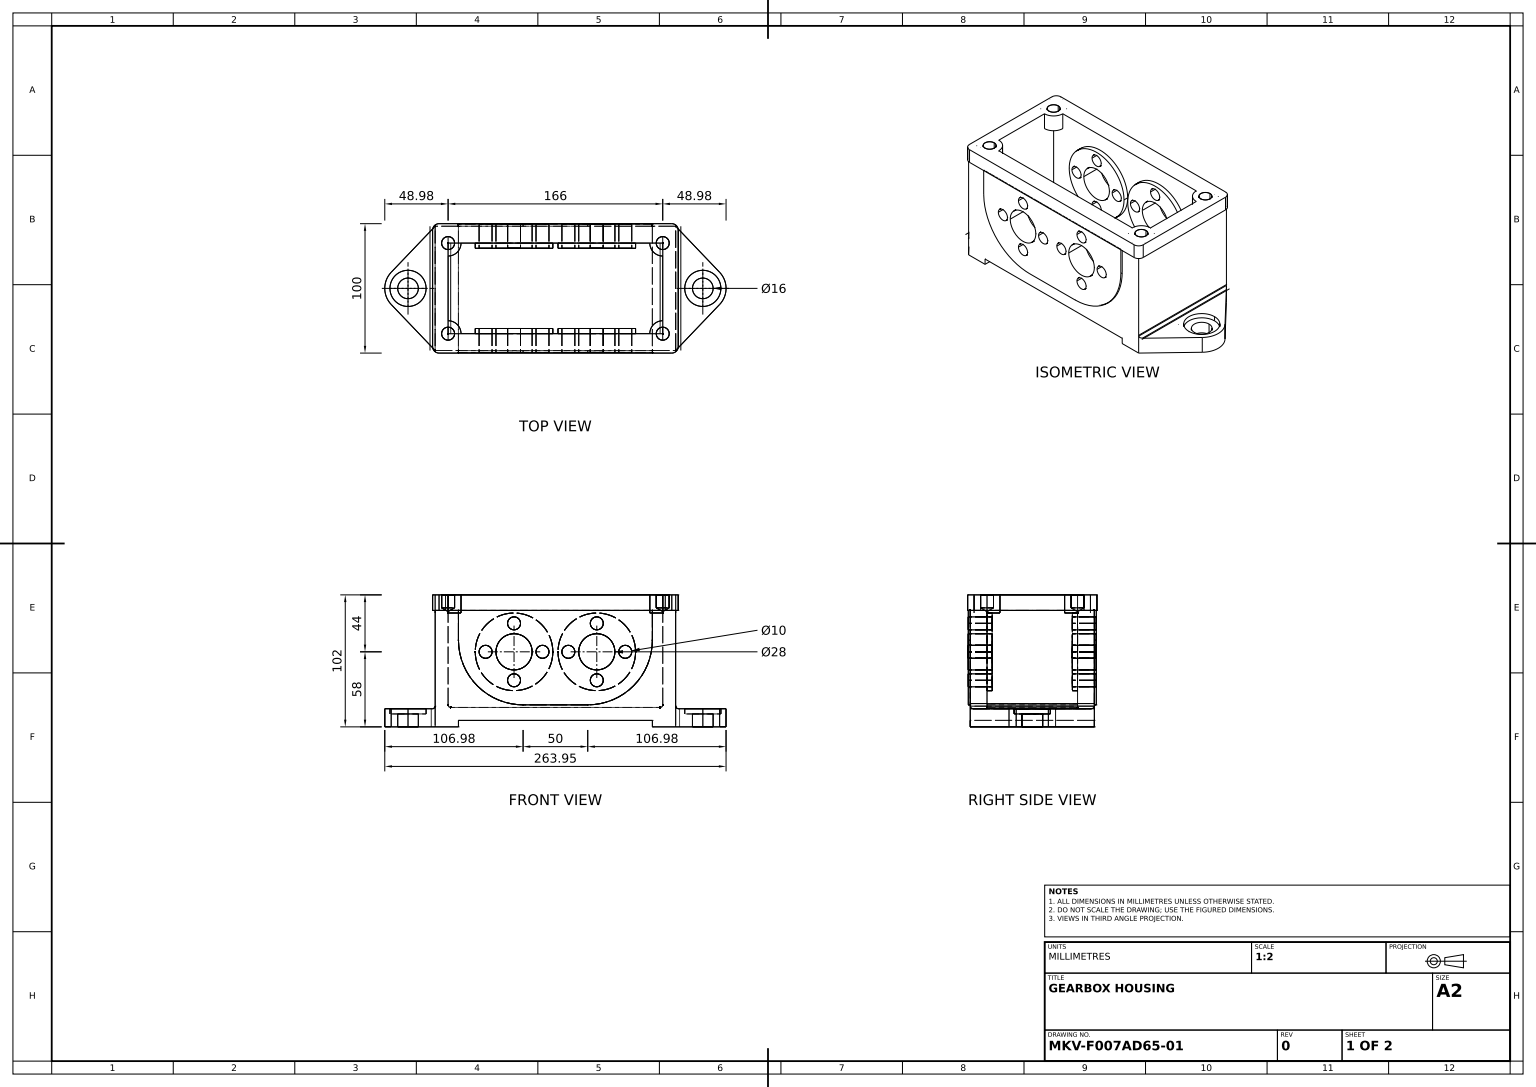
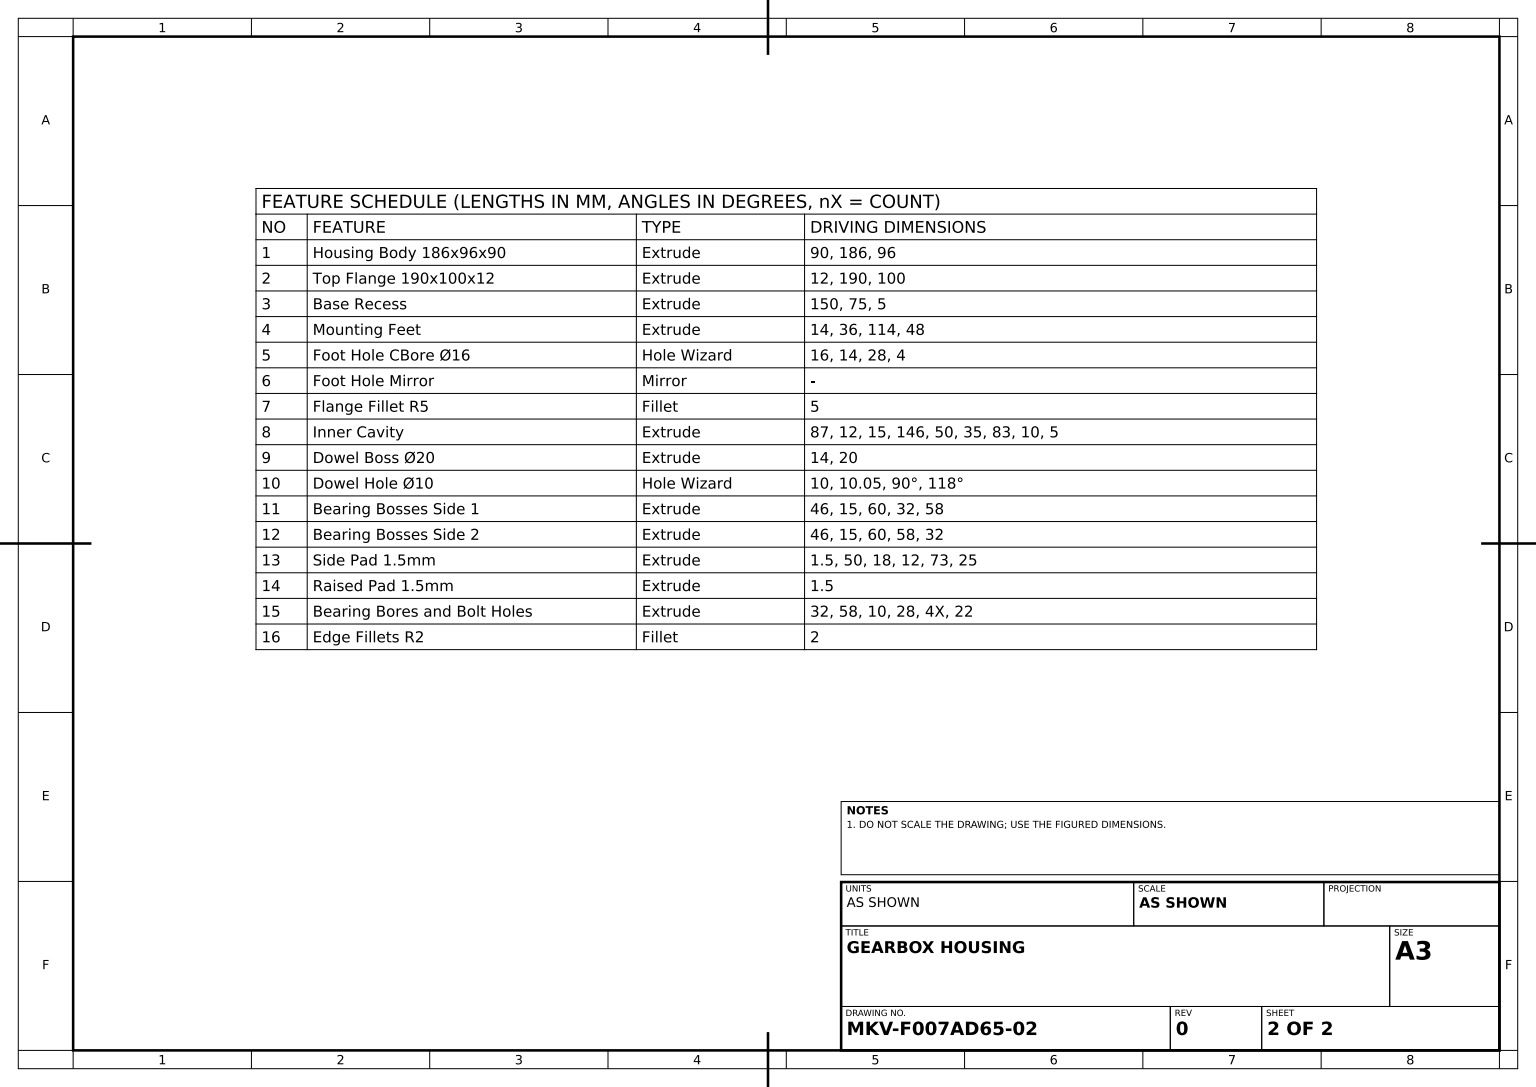
from build123d import *

# Parameters (mm, degrees)
HOUSING_BODY_SKETCH_W                   = 186
HOUSING_BODY_SKETCH_H                   = 96
HOUSING_BODY_186X96X90_DEPTH            = 90
TOP_FLANGE_SKETCH_W                     = 190
TOP_FLANGE_SKETCH_H                     = 100
TOP_FLANGE_190X100X12_DEPTH             = 12
BASE_RECESS_SKETCH_W                    = 150
BASE_RECESS_SKETCH_H                    = 5
BASE_RECESS_DEPTH                       = 171.390727447
MOUNTING_FEET_DEPTH                     = 14
FOOT_HOLE_CBORE_16_D                    = 16
FOOT_HOLE_CBORE_16_CBORE_D              = 28
FOOT_HOLE_CBORE_16_CBORE_DEPTH          = 4
FLANGE_FILLET_R5_R                      = 5
INNER_CAVITY_DEPTH                      = 87
DOWEL_BOSS_SKETCH_R                     = 10
DOWEL_BOSS_20_DEPTH                     = 14
DOWEL_HOLE_10_D                         = 10
DOWEL_HOLE_10_DEPTH                     = 10
DOWEL_HOLE_10_CSINK_D                   = 10.05
DOWEL_HOLE_10_CSINK_ANGLE               = 90
DOWEL_HOLE_10_TIP                       = 3.004303095
BEARING_BOSSES_SIDE_1_SKETCH_R          = 30
BEARING_BOSSES_SIDE_1_DEPTH             = 15
BEARING_START                           = -15
BEARING_BOSSES_SIDE_2_SKETCH_R          = 30
BEARING_BOSSES_SIDE_2_DEPTH             = 15
SIDE_PAD_1_5MM_DEPTH                    = 1.5
RAISED_START                            = 1.5
RAISED_PAD_1_5MM_DEPTH                  = 1.5
BEARING_BORES_AND_BOLT_HOLES_SKETCH_R   = 5
BEARING_BORES_AND_BOLT_HOLES_SKETCH_R_2 = 14
BEARING_BORES_AND_BOLT_HOLES_DEPTH      = 195.237612218
EDGE_FILLETS_R2_R                       = 2


with BuildPart() as part:
    # Housing Body Sketch → Housing Body 186x96x90 (new body)
    with BuildSketch(Plane(origin=(0, 0, 0), x_dir=(1, 0, 0), z_dir=(0, 1, 0))):
        Rectangle(HOUSING_BODY_SKETCH_W, HOUSING_BODY_SKETCH_H)
    extrude(amount=HOUSING_BODY_186X96X90_DEPTH)

    # Top Flange Sketch → Top Flange 190x100x12 (add)
    with BuildSketch(Plane(origin=(0, 90, 0), x_dir=(1, 0, 0), z_dir=(0, 1, 0))):
        Rectangle(TOP_FLANGE_SKETCH_W, TOP_FLANGE_SKETCH_H)
    extrude(amount=TOP_FLANGE_190X100X12_DEPTH)

    # Base Recess Sketch → Base Recess (cut, through all)
    with BuildSketch(Plane.XY.offset(48)):
        with Locations((0, 2.5)):
            Rectangle(BASE_RECESS_SKETCH_W, BASE_RECESS_SKETCH_H)
    extrude(amount=-BASE_RECESS_DEPTH, mode=Mode.SUBTRACT)

    # Mounting Feet Sketch → Mounting Feet (add)
    with BuildSketch(Plane.XZ):
        with BuildLine():
            Line((-127.008364611, 12.441159517), (-93, 48))
            Line((-93, 48), (-93, -48))
            Line((-93, -48), (-127.008364611, -12.441159517))
            ThreePointArc((-127.008364611, -12.441159517), (-132, 0), (-127.008364611, 12.441159517))
        make_face()
    mounting_feet = extrude(amount=-MOUNTING_FEET_DEPTH)

    # Foot Hole CBore Ø16 (through all)
    with Locations(Plane(origin=(0, 14, 0), x_dir=(1, 0, 0), z_dir=(0, 1, 0))):
        with Locations((-114, 0)):
            foot_hole_cbore_16 = CounterBoreHole(FOOT_HOLE_CBORE_16_D / 2, FOOT_HOLE_CBORE_16_CBORE_D / 2, FOOT_HOLE_CBORE_16_CBORE_DEPTH)

    # Foot Hole Mirror: Mounting Feet, Foot Hole CBore Ø16 across plane
    add(mounting_feet.mirror(Plane(origin=(0, 0, 0), x_dir=(0, 0, 1), z_dir=(1, 0, 0))))
    add(foot_hole_cbore_16.mirror(Plane(origin=(0, 0, 0), x_dir=(0, 0, 1), z_dir=(1, 0, 0))), mode=Mode.SUBTRACT)

    # Flange Fillet R5
    flange_fillet_r5_edges = [part.edges().sort_by_distance(p)[0] for p in [
        (95, 96, 50),
        (95, 96, -50),
        (-95, 96, -50),
        (-95, 96, 50),
    ]]
    fillet(flange_fillet_r5_edges, radius=FLANGE_FILLET_R5_R)

    # Inner Cavity Sketch → Inner Cavity (cut)
    with BuildSketch(Plane(origin=(0, 102, 0), x_dir=(1, 0, 0), z_dir=(0, 1, 0))):
        Polygon((-73, 35), (73, 35), (83, 35), (83, 25), (83, -25), (83, -35), (73, -35), (-73, -35), (-83, -35), (-83, -25), (-83, 25), (-83, 35), align=None)
    extrude(amount=-INNER_CAVITY_DEPTH, mode=Mode.SUBTRACT)

    # Dowel Boss Sketch → Dowel Boss Ø20 (add)
    with BuildSketch(Plane(origin=(0, 102, 0), x_dir=(1, 0, 0), z_dir=(0, 1, 0))):
        with Locations((-83, 35)):
            Circle(DOWEL_BOSS_SKETCH_R)
        with Locations((83, 35)):
            Circle(DOWEL_BOSS_SKETCH_R)
        with Locations((83, -35)):
            Circle(DOWEL_BOSS_SKETCH_R)
        with Locations((-83, -35)):
            Circle(DOWEL_BOSS_SKETCH_R)
    extrude(amount=-DOWEL_BOSS_20_DEPTH)

    # Dowel Hole Ø10
    with Locations(Plane(origin=(0, 102, 0), x_dir=(1, 0, 0), z_dir=(0, 1, 0))):
        with Locations((-83, -35), (-83, 35), (83, 35), (83, -35)):
            CounterSinkHole(DOWEL_HOLE_10_D / 2, DOWEL_HOLE_10_CSINK_D / 2, depth=DOWEL_HOLE_10_DEPTH, counter_sink_angle=DOWEL_HOLE_10_CSINK_ANGLE)
            with Locations((0, 0, -(DOWEL_HOLE_10_DEPTH + DOWEL_HOLE_10_TIP / 2))):  # 118° drill point
                Cone(0, DOWEL_HOLE_10_D / 2, DOWEL_HOLE_10_TIP, mode=Mode.SUBTRACT)

    # Bearing Bosses Side 1 Sketch → Bearing Bosses Side 1 (add)
    with BuildSketch(Plane.XY.offset(-46)):
        with Locations(Location((-32, 58, 0), (0, 0, 180))):
            Circle(BEARING_BOSSES_SIDE_1_SKETCH_R)
        with Locations(Location((32, 58, 0), (0, 0, 180))):
            Circle(BEARING_BOSSES_SIDE_1_SKETCH_R)
    extrude(amount=BEARING_BOSSES_SIDE_1_DEPTH)

    # Bearing Bosses Side 2 Sketch → Bearing Bosses Side 2 (add)
    with BuildSketch(Plane.XY.offset(46).offset(BEARING_START)):
        with Locations(Location((32, 58, 0), (0, 0, 180))):
            Circle(BEARING_BOSSES_SIDE_2_SKETCH_R)
        with Locations(Location((-32, 58, 0), (0, 0, 180))):
            Circle(BEARING_BOSSES_SIDE_2_SKETCH_R)
    extrude(amount=BEARING_BOSSES_SIDE_2_DEPTH)

    # Side Pad Sketch → Side Pad 1.5mm (add)
    with BuildSketch(Plane(origin=(0, 0, -48), x_dir=(-1, 0, 0), z_dir=(0, 0, -1))):
        with BuildLine():
            Line((-25, 17), (0, 17))
            Line((0, 17), (25, 17))
            ThreePointArc((25, 17), (60.355339059, 31.644660941), (75, 67))
            Line((75, 67), (75, 90))
            Line((75, 90), (-75, 90))
            Line((-75, 90), (-75, 67))
            ThreePointArc((-75, 67), (-60.355339059, 31.644660941), (-25, 17))
        make_face()
    extrude(amount=SIDE_PAD_1_5MM_DEPTH)

    # Raised Pad Sketch → Raised Pad 1.5mm (add)
    with BuildSketch(Plane.XY.offset(48).offset(RAISED_START)):
        with BuildLine():
            Line((75, 90), (75, 67))
            ThreePointArc((75, 67), (60.355339059, 31.644660941), (25, 17))
            Line((25, 17), (-25, 17))
            ThreePointArc((-25, 17), (-60.355339059, 31.644660941), (-75, 67))
            Line((-75, 67), (-75, 90))
            Line((-75, 90), (75, 90))
        make_face()
    extrude(amount=-RAISED_PAD_1_5MM_DEPTH)

    # Bearing Bores and Bolt Holes Sketch → Bearing Bores and Bolt Holes (cut, through all)
    with BuildSketch(Plane.XY.offset(49.5)):
        with Locations((-32, 80)):
            Circle(BEARING_BORES_AND_BOLT_HOLES_SKETCH_R)
        with Locations((32, 80)):
            Circle(BEARING_BORES_AND_BOLT_HOLES_SKETCH_R)
        with Locations((-32, 58)):
            Circle(BEARING_BORES_AND_BOLT_HOLES_SKETCH_R_2)
        with Locations((32, 58)):
            Circle(BEARING_BORES_AND_BOLT_HOLES_SKETCH_R_2)
        with Locations((-10, 58)):
            Circle(BEARING_BORES_AND_BOLT_HOLES_SKETCH_R)
        with Locations((-32, 36)):
            Circle(BEARING_BORES_AND_BOLT_HOLES_SKETCH_R)
        with Locations((-54, 58)):
            Circle(BEARING_BORES_AND_BOLT_HOLES_SKETCH_R)
        with Locations((54, 58)):
            Circle(BEARING_BORES_AND_BOLT_HOLES_SKETCH_R)
        with Locations((32, 36)):
            Circle(BEARING_BORES_AND_BOLT_HOLES_SKETCH_R)
        with Locations((10, 58)):
            Circle(BEARING_BORES_AND_BOLT_HOLES_SKETCH_R)
    extrude(amount=-BEARING_BORES_AND_BOLT_HOLES_DEPTH, mode=Mode.SUBTRACT)

    # Edge Fillets R2
    edge_fillets_r2_edges = [part.edges().sort_by_distance(p)[0] for p in [
        (83, 15, 0),
        (-83, 15, 0),
        (-93, 14, 0),
        (93, 14, 0),
    ]]
    fillet(edge_fillets_r2_edges, radius=EDGE_FILLETS_R2_R)


solid = part.part
